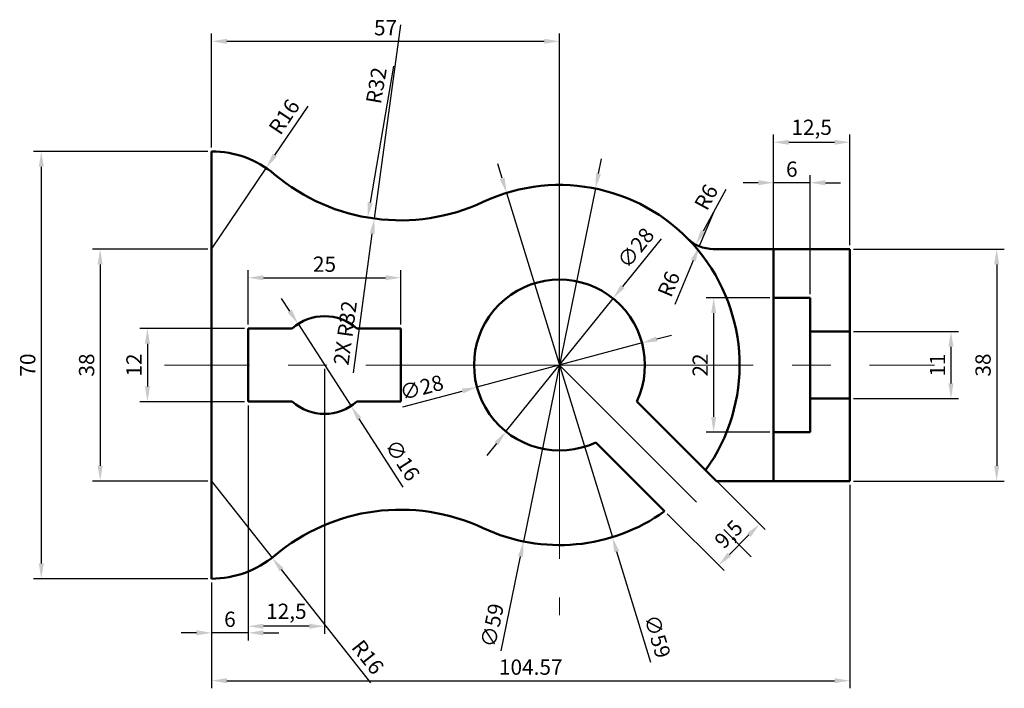
# Model space of a CAD drawing. Units: millimetres. Extents: x 3399 to 3560, y 1676 to 1786.
import ezdxf

# ---------------------------------------------------------------- set-up
doc = ezdxf.new("R2010")
doc.units = ezdxf.units.MM
doc.linetypes.add('CENTER', pattern=[50.8, 31.75, -6.35, 6.35, -6.35])
for name, color, linetype, lineweight in [('M-CNTR', 2, 'CENTER', 18), ('M-DIMS', 6, 'Continuous', 25), ('M-OUTL', 7, 'Continuous', 50)]:
    doc.layers.add(name, color=color, linetype=linetype, lineweight=lineweight)
doc.styles.get("Standard").update_dxf_attribs({"font": 'arial.ttf'})
doc.dimstyles.new('ISO-25', dxfattribs={"dimtxt": 2.5, "dimasz": 2.5, "dimexe": 1.25, "dimexo": 0.625, "dimtad": 1, "dimtxsty": 'Standard', "dimcen": 2.5, "dimadec": 0, "dimazin": 0, "dimtfac": 1, "dimtmove": 0, "dimatfit": 3, "dimfxl": 1, "dimarcsym": 0})

# ---------------------------------------------------------------- blocks, each defined once
blk = doc.blocks.new('*D1')
at = {"layer": 'Defpoints', "color": 0, "transparency": 16777216}
for p in [(3430.34, 1764.16), (3402.43, 1694.16), (3430.34, 1694.16)]:
    blk.add_point(p, dxfattribs=at)
at = {"layer": 'M-DIMS', "color": 0, "lineweight": -2, "transparency": 16777216}
for p, q in [((3429.72, 1764.16), (3401.18, 1764.16)), ((3402.43, 1761.66), (3402.43, 1696.66)), ((3429.72, 1694.16), (3401.18, 1694.16))]:
    blk.add_line(p, q, dxfattribs=at)
at = {"layer": 'M-DIMS', "color": 0, "transparency": 16777216}
for points in [[(3402.02, 1761.66), (3402.85, 1761.66), (3402.43, 1764.16)], [(3402.02, 1696.66), (3402.85, 1696.66), (3402.43, 1694.16)]]:
    blk.add_solid(points, dxfattribs=at)
at = {"layer": 'M-DIMS', "color": 0, "transparency": 16777216, "insert": (3400.53, 1729.16), "char_height": 2.5, "attachment_point": 5, "rotation": 90}
blk.add_mtext('70', dxfattribs=at)
blk = doc.blocks.new('*D2')
at = {"layer": 'Defpoints', "color": 0, "transparency": 16777216}
for p in [(3534.91, 1748.16), (3534.91, 1710.16), (3558.98, 1710.16)]:
    blk.add_point(p, dxfattribs=at)
at = {"layer": 'M-DIMS', "color": 0, "lineweight": -2, "transparency": 16777216}
for p, q in [((3535.53, 1748.16), (3560.23, 1748.16)), ((3558.98, 1745.66), (3558.98, 1712.66)), ((3535.53, 1710.16), (3560.23, 1710.16))]:
    blk.add_line(p, q, dxfattribs=at)
at = {"layer": 'M-DIMS', "color": 0, "transparency": 16777216}
for points in [[(3558.56, 1745.66), (3559.39, 1745.66), (3558.98, 1748.16)], [(3558.56, 1712.66), (3559.39, 1712.66), (3558.98, 1710.16)]]:
    blk.add_solid(points, dxfattribs=at)
at = {"layer": 'M-DIMS', "color": 0, "transparency": 16777216, "insert": (3557.07, 1729.16), "char_height": 2.5, "attachment_point": 5, "rotation": 90}
blk.add_mtext('38', dxfattribs=at)
blk = doc.blocks.new('*D3')
at = {"layer": 'Defpoints', "color": 0, "transparency": 16777216}
for p in [(3534.91, 1734.66), (3534.91, 1723.66), (3551.48, 1723.66)]:
    blk.add_point(p, dxfattribs=at)
at = {"layer": 'M-DIMS', "color": 0, "lineweight": -2, "transparency": 16777216}
for p, q in [((3535.53, 1734.66), (3552.73, 1734.66)), ((3551.48, 1732.16), (3551.48, 1726.16)), ((3535.53, 1723.66), (3552.73, 1723.66))]:
    blk.add_line(p, q, dxfattribs=at)
at = {"layer": 'M-DIMS', "color": 0, "transparency": 16777216}
for points in [[(3551.06, 1732.16), (3551.9, 1732.16), (3551.48, 1734.66)], [(3551.06, 1726.16), (3551.9, 1726.16), (3551.48, 1723.66)]]:
    blk.add_solid(points, dxfattribs=at)
at = {"layer": 'M-DIMS', "color": 0, "transparency": 16777216, "insert": (3549.6, 1729.16), "char_height": 2.5, "attachment_point": 5, "rotation": 90}
blk.add_mtext('11', dxfattribs=at)
blk = doc.blocks.new('*D4')
at = {"layer": 'Defpoints', "color": 0, "transparency": 16777216}
for p in [(3522.41, 1740.16), (3512.6, 1718.16), (3522.41, 1718.16)]:
    blk.add_point(p, dxfattribs=at)
at = {"layer": 'M-DIMS', "color": 0, "lineweight": -2, "transparency": 16777216}
for p, q in [((3521.78, 1740.16), (3511.35, 1740.16)), ((3512.6, 1737.66), (3512.6, 1720.66)), ((3521.78, 1718.16), (3511.35, 1718.16))]:
    blk.add_line(p, q, dxfattribs=at)
at = {"layer": 'M-DIMS', "color": 0, "transparency": 16777216}
for points in [[(3512.19, 1737.66), (3513.02, 1737.66), (3512.6, 1740.16)], [(3512.19, 1720.66), (3513.02, 1720.66), (3512.6, 1718.16)]]:
    blk.add_solid(points, dxfattribs=at)
at = {"layer": 'M-DIMS', "color": 0, "transparency": 16777216, "insert": (3510.72, 1729.16), "char_height": 2.5, "attachment_point": 5, "rotation": 90}
blk.add_mtext('22', dxfattribs=at)
blk = doc.blocks.new('*D5')
at = {"layer": 'Defpoints', "color": 0, "transparency": 16777216}
for p in [(3522.41, 1759.03), (3522.41, 1740.16), (3528.41, 1740.16)]:
    blk.add_point(p, dxfattribs=at)
at = {"layer": 'M-DIMS', "color": 0, "lineweight": -2, "transparency": 16777216}
for p, q in [((3522.41, 1740.79), (3522.41, 1760.28)), ((3528.41, 1740.79), (3528.41, 1760.28)), ((3519.91, 1759.03), (3517.41, 1759.03)), ((3528.41, 1759.03), (3522.41, 1759.03)), ((3530.91, 1759.03), (3533.41, 1759.03))]:
    blk.add_line(p, q, dxfattribs=at)
at = {"layer": 'M-DIMS', "color": 0, "transparency": 16777216}
for points in [[(3519.91, 1759.45), (3519.91, 1758.61), (3522.41, 1759.03)], [(3530.91, 1759.45), (3530.91, 1758.61), (3528.41, 1759.03)]]:
    blk.add_solid(points, dxfattribs=at)
at = {"layer": 'M-DIMS', "color": 0, "transparency": 16777216, "insert": (3525.41, 1760.93), "char_height": 2.5, "attachment_point": 5}
blk.add_mtext('6', dxfattribs=at)
blk = doc.blocks.new('*D6')
at = {"layer": 'Defpoints', "color": 0, "transparency": 16777216}
for p in [(3511.29, 1711.93), (3504.57, 1705.22), (3513.42, 1696.37)]:
    blk.add_point(p, dxfattribs=at)
at = {"layer": 'M-DIMS', "color": 0, "lineweight": -2, "transparency": 16777216}
for p, q in [((3511.73, 1711.49), (3521.02, 1702.2)), ((3505.01, 1704.78), (3514.3, 1695.48)), ((3518.37, 1701.32), (3515.19, 1698.14))]:
    blk.add_line(p, q, dxfattribs=at)
at = {"layer": 'M-DIMS', "color": 0, "transparency": 16777216}
for points in [[(3518.08, 1701.61), (3518.66, 1701.02), (3520.14, 1703.09)], [(3514.89, 1698.43), (3515.48, 1697.84), (3513.42, 1696.37)]]:
    blk.add_solid(points, dxfattribs=at)
at = {"layer": 'M-DIMS', "color": 0, "transparency": 16777216, "insert": (3515.28, 1701.23), "char_height": 2.5, "attachment_point": 5, "rotation": 45}
blk.add_mtext('9,5', dxfattribs=at)
blk = doc.blocks.new('*D7')
at = {"layer": 'Defpoints', "color": 0, "transparency": 16777216}
for p in [(3439.27, 1761.44), (3430.34, 1748.16)]:
    blk.add_point(p, dxfattribs=at)
at = {"layer": 'M-DIMS', "color": 0, "lineweight": -2, "transparency": 16777216}
for p, q in [((3446.09, 1771.58), (3440.66, 1763.52)), ((3430.34, 1748.16), (3439.27, 1761.44))]:
    blk.add_line(p, q, dxfattribs=at)
at = {"layer": 'M-DIMS', "color": 0, "transparency": 16777216}
blk.add_solid([(3440.32, 1763.75), (3441.01, 1763.28), (3439.27, 1761.44)], dxfattribs=at)
at = {"layer": 'M-DIMS', "color": 0, "transparency": 16777216, "insert": (3442.5, 1769.65), "char_height": 2.5, "attachment_point": 5, "rotation": 56.0827}
blk.add_mtext('R16', dxfattribs=at)
blk = doc.blocks.new('*D8')
at = {"layer": 'Defpoints', "color": 0, "transparency": 16777216}
for p in [(3430.34, 1710.16), (3440.25, 1697.6)]:
    blk.add_point(p, dxfattribs=at)
at = {"layer": 'M-DIMS', "color": 0, "lineweight": -2, "transparency": 16777216}
for p, q in [((3430.34, 1710.16), (3440.25, 1697.6)), ((3456.43, 1677.1), (3441.8, 1695.64))]:
    blk.add_line(p, q, dxfattribs=at)
at = {"layer": 'M-DIMS', "color": 0, "transparency": 16777216}
blk.add_solid([(3442.13, 1695.9), (3441.47, 1695.38), (3440.25, 1697.6)], dxfattribs=at)
at = {"layer": 'M-DIMS', "color": 0, "transparency": 16777216, "insert": (3455.69, 1681.11), "char_height": 2.5, "attachment_point": 5, "rotation": 308.2765}
blk.add_mtext('R16', dxfattribs=at)
blk = doc.blocks.new('*D9')
at = {"layer": 'Defpoints', "color": 0, "transparency": 16777216}
for p in [(3461.28, 1784.87), (3455.9, 1753.32)]:
    blk.add_point(p, dxfattribs=at)
at = {"layer": 'M-DIMS', "color": 0, "lineweight": -2, "transparency": 16777216}
blk.add_line((3460.13, 1778.13), (3456.32, 1755.79), dxfattribs=at)
at = {"layer": 'M-DIMS', "color": 0, "transparency": 16777216}
blk.add_solid([(3455.91, 1755.86), (3456.73, 1755.72), (3455.9, 1753.32)], dxfattribs=at)
at = {"layer": 'M-DIMS', "color": 0, "transparency": 16777216, "insert": (3457.65, 1774.9), "char_height": 2.5, "attachment_point": 5, "rotation": 80.3303}
blk.add_mtext('R32', dxfattribs=at)
blk = doc.blocks.new('*D10')
at = {"layer": 'Defpoints', "color": 0, "transparency": 16777216}
for p in [(3512.55, 1754.16), (3509.67, 1748.9)]:
    blk.add_point(p, dxfattribs=at)
at = {"layer": 'M-DIMS', "color": 0, "lineweight": -2, "transparency": 16777216}
blk.add_line((3514.6, 1757.92), (3510.87, 1751.09), dxfattribs=at)
at = {"layer": 'M-DIMS', "color": 0, "transparency": 16777216}
blk.add_solid([(3510.5, 1751.29), (3511.23, 1750.89), (3509.67, 1748.9)], dxfattribs=at)
at = {"layer": 'M-DIMS', "color": 0, "transparency": 16777216, "insert": (3511.66, 1756.51), "char_height": 2.5, "attachment_point": 5, "rotation": 61.3621}
blk.add_mtext('R6', dxfattribs=at)
blk = doc.blocks.new('*D11')
at = {"layer": 'Defpoints', "color": 0, "transparency": 16777216}
for p in [(3444.51, 1735.89), (3453.18, 1722.44)]:
    blk.add_point(p, dxfattribs=at)
at = {"layer": 'M-DIMS', "color": 0, "lineweight": -2, "transparency": 16777216}
for p, q in [((3443.15, 1737.99), (3441.8, 1740.09)), ((3444.51, 1735.89), (3453.18, 1722.44)), ((3461.73, 1709.17), (3454.53, 1720.34))]:
    blk.add_line(p, q, dxfattribs=at)
at = {"layer": 'M-DIMS', "color": 0, "transparency": 16777216}
for points in [[(3443.5, 1738.21), (3442.8, 1737.76), (3444.51, 1735.89)], [(3454.88, 1720.56), (3454.18, 1720.11), (3453.18, 1722.44)]]:
    blk.add_solid(points, dxfattribs=at)
at = {"layer": 'M-DIMS', "color": 0, "transparency": 16777216, "insert": (3461.34, 1713.41), "char_height": 2.5, "attachment_point": 5, "rotation": 302.8035}
blk.add_mtext('∅16', dxfattribs=at)
blk = doc.blocks.new('*D12')
at = {"layer": 'Defpoints', "color": 0, "transparency": 16777216}
for p in [(3496.11, 1740.07), (3478.57, 1718.25)]:
    blk.add_point(p, dxfattribs=at)
at = {"layer": 'M-DIMS', "color": 0, "lineweight": -2, "transparency": 16777216}
for p, q in [((3503.98, 1749.86), (3497.68, 1742.02)), ((3478.57, 1718.25), (3496.11, 1740.07)), ((3477, 1716.3), (3475.44, 1714.36))]:
    blk.add_line(p, q, dxfattribs=at)
at = {"layer": 'M-DIMS', "color": 0, "transparency": 16777216}
for points in [[(3497.36, 1742.28), (3498.01, 1741.76), (3496.11, 1740.07)], [(3476.68, 1716.57), (3477.33, 1716.04), (3478.57, 1718.25)]]:
    blk.add_solid(points, dxfattribs=at)
at = {"layer": 'M-DIMS', "color": 0, "transparency": 16777216, "insert": (3500.08, 1748.15), "char_height": 2.5, "attachment_point": 5, "rotation": 51.2016}
blk.add_mtext('∅28', dxfattribs=at)
blk = doc.blocks.new('*D13')
at = {"layer": 'Defpoints', "color": 0, "transparency": 16777216}
for p in [(3493.23, 1758.07), (3481.46, 1700.26)]:
    blk.add_point(p, dxfattribs=at)
at = {"layer": 'M-DIMS', "color": 0, "lineweight": -2, "transparency": 16777216}
for p, q in [((3493.73, 1760.52), (3494.22, 1762.97)), ((3493.23, 1758.07), (3481.46, 1700.26)), ((3477.81, 1682.36), (3480.96, 1697.81))]:
    blk.add_line(p, q, dxfattribs=at)
at = {"layer": 'M-DIMS', "color": 0, "transparency": 16777216}
for points in [[(3493.32, 1760.6), (3494.13, 1760.44), (3493.23, 1758.07)], [(3480.55, 1697.89), (3481.37, 1697.72), (3481.46, 1700.26)]]:
    blk.add_solid(points, dxfattribs=at)
at = {"layer": 'M-DIMS', "color": 0, "transparency": 16777216, "insert": (3476.63, 1686.45), "char_height": 2.5, "attachment_point": 5, "rotation": 78.4924}
blk.add_mtext('∅59', dxfattribs=at)
blk = doc.blocks.new('*D14')
at = {"layer": 'Defpoints', "color": 0, "transparency": 16777216}
for p in [(3461.34, 1743.46), (3436.34, 1735.16), (3461.34, 1735.16)]:
    blk.add_point(p, dxfattribs=at)
at = {"layer": 'M-DIMS', "color": 0, "lineweight": -2, "transparency": 16777216}
for p, q in [((3436.34, 1735.79), (3436.34, 1744.71)), ((3461.34, 1735.79), (3461.34, 1744.71)), ((3438.84, 1743.46), (3458.84, 1743.46))]:
    blk.add_line(p, q, dxfattribs=at)
at = {"layer": 'M-DIMS', "color": 0, "transparency": 16777216}
for points in [[(3438.84, 1743.88), (3438.84, 1743.04), (3436.34, 1743.46)], [(3458.84, 1743.88), (3458.84, 1743.04), (3461.34, 1743.46)]]:
    blk.add_solid(points, dxfattribs=at)
at = {"layer": 'M-DIMS', "color": 0, "transparency": 16777216, "insert": (3448.84, 1745.36), "char_height": 2.5, "attachment_point": 5}
blk.add_mtext('25', dxfattribs=at)
blk = doc.blocks.new('*D15')
at = {"layer": 'Defpoints', "color": 0, "transparency": 16777216}
for p in [(3430.34, 1748.16), (3412.08, 1710.16), (3430.34, 1710.16)]:
    blk.add_point(p, dxfattribs=at)
at = {"layer": 'M-DIMS', "color": 0, "lineweight": -2, "transparency": 16777216}
for p, q in [((3429.72, 1748.16), (3410.83, 1748.16)), ((3412.08, 1745.66), (3412.08, 1712.66)), ((3429.72, 1710.16), (3410.83, 1710.16))]:
    blk.add_line(p, q, dxfattribs=at)
at = {"layer": 'M-DIMS', "color": 0, "transparency": 16777216}
for points in [[(3411.66, 1745.66), (3412.49, 1745.66), (3412.08, 1748.16)], [(3411.66, 1712.66), (3412.49, 1712.66), (3412.08, 1710.16)]]:
    blk.add_solid(points, dxfattribs=at)
at = {"layer": 'M-DIMS', "color": 0, "transparency": 16777216, "insert": (3410.18, 1729.16), "char_height": 2.5, "attachment_point": 5, "rotation": 90}
blk.add_mtext('38', dxfattribs=at)
blk = doc.blocks.new('*D16')
at = {"layer": 'Defpoints', "color": 0, "transparency": 16777216}
for p in [(3436.34, 1735.16), (3419.82, 1723.16), (3436.34, 1723.16)]:
    blk.add_point(p, dxfattribs=at)
at = {"layer": 'M-DIMS', "color": 0, "lineweight": -2, "transparency": 16777216}
for p, q in [((3435.72, 1735.16), (3418.57, 1735.16)), ((3419.82, 1732.66), (3419.82, 1725.66)), ((3435.72, 1723.16), (3418.57, 1723.16))]:
    blk.add_line(p, q, dxfattribs=at)
at = {"layer": 'M-DIMS', "color": 0, "transparency": 16777216}
for points in [[(3419.41, 1732.66), (3420.24, 1732.66), (3419.82, 1735.16)], [(3419.41, 1725.66), (3420.24, 1725.66), (3419.82, 1723.16)]]:
    blk.add_solid(points, dxfattribs=at)
at = {"layer": 'M-DIMS', "color": 0, "transparency": 16777216, "insert": (3417.94, 1729.16), "char_height": 2.5, "attachment_point": 5, "rotation": 90}
blk.add_mtext('12', dxfattribs=at)
blk = doc.blocks.new('*D17')
at = {"layer": 'Defpoints', "color": 0, "transparency": 16777216}
for p in [(3487.34, 1782.2), (3430.34, 1764.16), (3487.34, 1729.16)]:
    blk.add_point(p, dxfattribs=at)
at = {"layer": 'M-DIMS', "color": 0, "lineweight": -2, "transparency": 16777216}
for p, q in [((3430.34, 1764.79), (3430.34, 1783.45)), ((3487.34, 1729.79), (3487.34, 1783.45)), ((3432.84, 1782.2), (3484.84, 1782.2))]:
    blk.add_line(p, q, dxfattribs=at)
at = {"layer": 'M-DIMS', "color": 0, "transparency": 16777216}
for points in [[(3432.84, 1782.62), (3432.84, 1781.78), (3430.34, 1782.2)], [(3484.84, 1782.62), (3484.84, 1781.78), (3487.34, 1782.2)]]:
    blk.add_solid(points, dxfattribs=at)
at = {"layer": 'M-DIMS', "color": 0, "transparency": 16777216, "insert": (3458.84, 1784.1), "char_height": 2.5, "attachment_point": 5}
blk.add_mtext('57', dxfattribs=at)
blk = doc.blocks.new('*D18')
at = {"layer": 'Defpoints', "color": 0, "transparency": 16777216}
for p in [(3436.34, 1723.16), (3430.34, 1694.16), (3430.34, 1685.29)]:
    blk.add_point(p, dxfattribs=at)
at = {"layer": 'M-DIMS', "color": 0, "lineweight": -2, "transparency": 16777216}
for p, q in [((3436.34, 1722.54), (3436.34, 1684.04)), ((3430.34, 1693.54), (3430.34, 1684.04)), ((3427.84, 1685.29), (3425.34, 1685.29)), ((3436.34, 1685.29), (3430.34, 1685.29)), ((3438.84, 1685.29), (3441.34, 1685.29))]:
    blk.add_line(p, q, dxfattribs=at)
at = {"layer": 'M-DIMS', "color": 0, "transparency": 16777216}
for points in [[(3427.84, 1685.71), (3427.84, 1684.88), (3430.34, 1685.29)], [(3438.84, 1685.71), (3438.84, 1684.88), (3436.34, 1685.29)]]:
    blk.add_solid(points, dxfattribs=at)
at = {"layer": 'M-DIMS', "color": 0, "transparency": 16777216, "insert": (3433.34, 1687.19), "char_height": 2.5, "attachment_point": 5}
blk.add_mtext('6', dxfattribs=at)
blk = doc.blocks.new('*D19')
at = {"layer": 'Defpoints', "color": 0, "transparency": 16777216}
for p in [(3448.84, 1729.16), (3436.34, 1723.16), (3436.34, 1686.37)]:
    blk.add_point(p, dxfattribs=at)
at = {"layer": 'M-DIMS', "color": 0, "lineweight": -2, "transparency": 16777216}
for p, q in [((3448.84, 1728.54), (3448.84, 1685.12)), ((3436.34, 1722.54), (3436.34, 1685.12)), ((3446.34, 1686.37), (3438.84, 1686.37))]:
    blk.add_line(p, q, dxfattribs=at)
at = {"layer": 'M-DIMS', "color": 0, "transparency": 16777216}
for points in [[(3438.84, 1686.79), (3438.84, 1685.95), (3436.34, 1686.37)], [(3446.34, 1686.79), (3446.34, 1685.95), (3448.84, 1686.37)]]:
    blk.add_solid(points, dxfattribs=at)
at = {"layer": 'M-DIMS', "color": 0, "transparency": 16777216, "insert": (3442.59, 1688.5), "char_height": 2.5, "attachment_point": 5}
blk.add_mtext('12,5', dxfattribs=at)
blk = doc.blocks.new('*D20')
at = {"layer": 'Defpoints', "color": 0, "transparency": 16777216}
for p in [(3534.91, 1765.66), (3534.91, 1748.16), (3522.41, 1740.16)]:
    blk.add_point(p, dxfattribs=at)
at = {"layer": 'M-DIMS', "color": 0, "lineweight": -2, "transparency": 16777216}
for p, q in [((3522.41, 1740.79), (3522.41, 1766.91)), ((3534.91, 1748.79), (3534.91, 1766.91)), ((3524.91, 1765.66), (3532.41, 1765.66))]:
    blk.add_line(p, q, dxfattribs=at)
at = {"layer": 'M-DIMS', "color": 0, "transparency": 16777216}
for points in [[(3524.91, 1766.07), (3524.91, 1765.24), (3522.41, 1765.66)], [(3532.41, 1766.07), (3532.41, 1765.24), (3534.91, 1765.66)]]:
    blk.add_solid(points, dxfattribs=at)
at = {"layer": 'M-DIMS', "color": 0, "transparency": 16777216, "insert": (3528.66, 1767.79), "char_height": 2.5, "attachment_point": 5}
blk.add_mtext('12,5', dxfattribs=at)
blk = doc.blocks.new('*D21')
at = {"layer": 'Defpoints', "color": 0, "transparency": 16777216}
for p in [(3534.91, 1710.16), (3430.34, 1694.16), (3534.91, 1677.45)]:
    blk.add_point(p, dxfattribs=at)
at = {"layer": 'M-DIMS', "color": 0, "lineweight": -2, "transparency": 16777216}
for p, q in [((3534.91, 1709.54), (3534.91, 1676.2)), ((3430.34, 1693.54), (3430.34, 1676.2)), ((3432.84, 1677.45), (3532.41, 1677.45))]:
    blk.add_line(p, q, dxfattribs=at)
at = {"layer": 'M-DIMS', "color": 0, "transparency": 16777216}
for points in [[(3432.84, 1677.87), (3432.84, 1677.04), (3430.34, 1677.45)], [(3532.41, 1677.87), (3532.41, 1677.04), (3534.91, 1677.45)]]:
    blk.add_solid(points, dxfattribs=at)
at = {"layer": 'M-DIMS', "color": 0, "transparency": 16777216, "insert": (3482.63, 1679.35), "char_height": 2.5, "attachment_point": 5}
blk.add_mtext('104.57', dxfattribs=at)
blk = doc.blocks.new('*D22')
at = {"layer": 'Defpoints', "color": 0, "transparency": 16777216}
for p in [(3478.68, 1757.36), (3496, 1700.96)]:
    blk.add_point(p, dxfattribs=at)
at = {"layer": 'M-DIMS', "color": 0, "lineweight": -2, "transparency": 16777216}
for p, q in [((3477.95, 1759.75), (3477.22, 1762.14)), ((3478.68, 1757.36), (3496, 1700.96)), ((3502.3, 1680.43), (3496.73, 1698.57))]:
    blk.add_line(p, q, dxfattribs=at)
at = {"layer": 'M-DIMS', "color": 0, "transparency": 16777216}
for points in [[(3478.35, 1759.88), (3477.55, 1759.63), (3478.68, 1757.36)], [(3497.13, 1698.69), (3496.33, 1698.45), (3496, 1700.96)]]:
    blk.add_solid(points, dxfattribs=at)
at = {"layer": 'M-DIMS', "color": 0, "transparency": 16777216, "insert": (3503.08, 1684.62), "char_height": 2.5, "attachment_point": 5, "rotation": 287.0655}
blk.add_mtext('∅59', dxfattribs=at)
blk = doc.blocks.new('*D23')
at = {"layer": 'Defpoints', "color": 0, "transparency": 16777216}
for p in [(3500.87, 1732.79), (3473.82, 1725.54)]:
    blk.add_point(p, dxfattribs=at)
at = {"layer": 'M-DIMS', "color": 0, "lineweight": -2, "transparency": 16777216}
for p, q in [((3500.87, 1732.79), (3473.82, 1725.54)), ((3503.28, 1733.43), (3505.69, 1734.08)), ((3461.69, 1722.29), (3471.4, 1724.89))]:
    blk.add_line(p, q, dxfattribs=at)
at = {"layer": 'M-DIMS', "color": 0, "transparency": 16777216}
for points in [[(3503.17, 1733.84), (3503.39, 1733.03), (3500.87, 1732.79)], [(3471.3, 1725.3), (3471.51, 1724.49), (3473.82, 1725.54)]]:
    blk.add_solid(points, dxfattribs=at)
at = {"layer": 'M-DIMS', "color": 0, "transparency": 16777216, "insert": (3464.83, 1725.17), "char_height": 2.5, "attachment_point": 5, "rotation": 14.9994}
blk.add_mtext('∅28', dxfattribs=at)
blk = doc.blocks.new('*D24')
at = {"layer": 'Defpoints', "color": 0, "transparency": 16777216}
for p in [(3461.28, 1784.87), (3457, 1753.15)]:
    blk.add_point(p, dxfattribs=at)
at = {"layer": 'M-DIMS', "color": 0, "lineweight": -2, "transparency": 16777216}
for p, q in [((3461.28, 1784.87), (3457, 1753.15)), ((3453.59, 1727.88), (3456.66, 1750.68))]:
    blk.add_line(p, q, dxfattribs=at)
at = {"layer": 'M-DIMS', "color": 0, "transparency": 16777216}
blk.add_solid([(3456.25, 1750.73), (3457.08, 1750.62), (3457, 1753.15)], dxfattribs=at)
at = {"layer": 'M-DIMS', "color": 0, "transparency": 16777216, "insert": (3452.55, 1734.38), "char_height": 2.5, "attachment_point": 5, "rotation": 82.3171}
blk.add_mtext('2X R32', dxfattribs=at)
blk = doc.blocks.new('*D25')
at = {"layer": 'Defpoints', "color": 0, "transparency": 16777216}
for p in [(3512.55, 1754.16), (3510.24, 1748.62)]:
    blk.add_point(p, dxfattribs=at)
at = {"layer": 'M-DIMS', "color": 0, "lineweight": -2, "transparency": 16777216}
for p, q in [((3512.55, 1754.16), (3510.24, 1748.62)), ((3506.29, 1739.14), (3509.28, 1746.32))]:
    blk.add_line(p, q, dxfattribs=at)
at = {"layer": 'M-DIMS', "color": 0, "transparency": 16777216}
blk.add_solid([(3508.89, 1746.48), (3509.66, 1746.16), (3510.24, 1748.62)], dxfattribs=at)
at = {"layer": 'M-DIMS', "color": 0, "transparency": 16777216, "insert": (3505.55, 1742.3), "char_height": 2.5, "attachment_point": 5, "rotation": 67.3845}
blk.add_mtext('R6', dxfattribs=at)

msp = doc.modelspace()

# ---------------------------------------------------------------- linework, layer by layer
at = {"layer": 'M-CNTR'}
for p, q in [((3487.342, 1729.164), (3487.342, 1768.619)), ((3430.342, 1729.164), (3422.595, 1729.164)), ((3487.342, 1729.164), (3430.342, 1729.164)), ((3487.342, 1729.164), (3521.362, 1695.143)), ((3487.342, 1729.164), (3548.781, 1729.164)), ((3487.342, 1729.164), (3487.342, 1688.203))]:
    msp.add_line(p, q, dxfattribs=at)
at = {"layer": 'M-OUTL'}
for p, q in [((3430.342, 1729.164), (3430.342, 1764.164)), ((3512.546, 1748.164), (3534.909, 1748.164)), ((3522.409, 1748.164), (3522.409, 1710.164)), ((3534.909, 1748.164), (3534.909, 1710.164)), ((3522.409, 1740.164), (3528.409, 1740.164)), ((3528.409, 1740.164), (3528.409, 1718.164)), ((3436.342, 1729.164), (3436.342, 1735.164)), ((3436.342, 1735.164), (3443.551, 1735.164)), ((3454.134, 1735.164), (3461.342, 1735.164)), ((3461.342, 1735.164), (3461.342, 1723.164)), ((3528.409, 1734.664), (3534.909, 1734.664)), ((3534.909, 1734.664), (3534.909, 1723.664)), ((3430.342, 1729.164), (3430.342, 1694.164)), ((3436.342, 1723.164), (3436.342, 1729.164)), ((3443.551, 1723.164), (3436.342, 1723.164)), ((3461.342, 1723.164), (3454.134, 1723.164)), ((3500.013, 1723.21), (3513.06, 1710.164)), ((3534.909, 1723.664), (3528.409, 1723.664)), ((3528.409, 1718.164), (3522.409, 1718.164)), ((3493.296, 1716.492), (3504.571, 1705.217)), ((3430.342, 1694.164), (3430.342, 1710.164)), ((3534.909, 1710.164), (3513.06, 1710.164))]:
    msp.add_line(p, q, dxfattribs=at)
for centre, radius, start, end in [((3430.342, 1748.164), 16, 49.87518, 90), ((3461.276, 1784.866), 32, 229.87518, 295.07726), ((3487.342, 1729.164), 29.5, 324.26593, 115.07726), ((3512.546, 1754.164), 6, 224.767, 270), ((3487.342, 1729.164), 14, 334.83336, 295.16664), ((3448.842, 1729.164), 8, 48.59038, 131.40962), ((3448.842, 1729.164), 8, 228.59038, 311.40962), ((3461.276, 1673.461), 32, 64.92274, 130.12482), ((3487.342, 1729.164), 29.5, 244.92274, 305.73407), ((3430.342, 1710.164), 16, 270, 310.12482)]:
    msp.add_arc(centre, radius, start, end, dxfattribs=at)

# ---------------------------------------------------------------- dimensions: what is measured, and where the dimension line sits
at = {"layer": 'M-DIMS'}
for base, p1, p2, override, picture, middle in [((3487.342, 1782.201), (3430.342, 1764.164), (3487.342, 1729.164), {"dimclrd": 0, "dimclre": 0, "dimclrt": 0}, '*D17', (3458.842, 1784.097)), ((3534.909, 1765.658), (3522.409, 1740.164), (3534.909, 1748.164), {"dimclrd": 0, "dimclre": 0, "dimclrt": 0}, '*D20', (3528.659, 1767.786)), ((3522.409, 1759.029), (3528.409, 1740.164), (3522.409, 1740.164), {"dimclrd": 0, "dimclre": 0, "dimclrt": 0}, '*D5', (3525.409, 1760.931)), ((3461.342, 1743.461), (3436.342, 1735.164), (3461.342, 1735.164), {"dimclrd": 0, "dimclre": 0, "dimclrt": 0}, '*D14', (3448.842, 1745.362)), ((3436.342, 1686.369), (3448.842, 1729.164), (3436.342, 1723.164), {"dimclrd": 0, "dimclre": 0, "dimclrt": 0}, '*D19', (3442.592, 1688.496)), ((3430.342, 1685.293), (3436.342, 1723.164), (3430.342, 1694.164), {"dimclrd": 0, "dimclre": 0, "dimclrt": 0}, '*D18', (3433.342, 1687.195)), ((3534.909, 1677.453), (3430.342, 1694.164), (3534.909, 1710.164), {"dimdec": 2, "dimlfac": 1, "dimrnd": 0, "dimzin": 0, "dimdsep": 46, "dimlunit": 2}, '*D21', (3482.625, 1679.354))]:
    dim = msp.add_linear_dim(base=base, p1=p1, p2=p2, dimstyle='ISO-25', override=override, dxfattribs=at)
    dim.commit()
    dim.dimension.update_dxf_attribs({"geometry": picture, "text_midpoint": middle})
dim = msp.add_radius_dim(center=(3461.276, 1784.866), mpoint=(3456.998, 1753.154), text='2X <>', dimstyle='ISO-25', override={"dimdec": 0, "dimlfac": 1, "dimrnd": 0, "dimzin": 0, "dimdsep": 46, "dimlunit": 2}, dxfattribs=at)
dim.commit()
dim.dimension.update_dxf_attribs({"geometry": '*D24', "text_midpoint": (3454.431, 1734.126), "dimtype": 164})
for center, mpoint, picture, middle in [((3461.276, 1784.866), (3455.901, 1753.321), '*D9', (3459.523, 1774.581)), ((3512.546, 1754.164), (3509.671, 1748.898), '*D10', (3513.332, 1755.603)), ((3430.342, 1710.164), (3440.253, 1697.603), '*D8', (3454.198, 1679.931))]:
    dim = msp.add_radius_dim(center=center, mpoint=mpoint, dimstyle='ISO-25', override={"dimclrd": 0, "dimclre": 0, "dimclrt": 0}, dxfattribs=at)
    dim.commit()
    dim.dimension.update_dxf_attribs({"geometry": picture, "text_midpoint": middle, "dimtype": 164})
for center, mpoint, override, picture, middle in [((3430.342, 1748.164), (3439.27, 1761.441), {"dimclrd": 0, "dimclre": 0, "dimclrt": 0}, '*D7', (3442.497, 1769.648)), ((3512.546, 1754.164), (3510.239, 1748.625), {"dimdec": 0, "dimlfac": 1, "dimrnd": 0, "dimzin": 0, "dimdsep": 46, "dimlunit": 2}, '*D25', (3505.546, 1742.304))]:
    dim = msp.add_radius_dim(center=center, mpoint=mpoint, dimstyle='ISO-25', override=override, dxfattribs=at)
    dim.commit()
    dim.dimension.update_dxf_attribs({"geometry": picture, "text_midpoint": middle})
for base, p1, p2, picture, middle in [((3402.434, 1694.164), (3430.342, 1764.164), (3430.342, 1694.164), '*D1', (3400.533, 1729.164)), ((3412.077, 1710.164), (3430.342, 1748.164), (3430.342, 1710.164), '*D15', (3410.175, 1729.164)), ((3558.977, 1710.164), (3534.909, 1748.164), (3534.909, 1710.164), '*D2', (3557.074, 1729.164)), ((3512.602, 1718.164), (3522.409, 1740.164), (3522.409, 1718.164), '*D4', (3510.722, 1729.164)), ((3419.824, 1723.164), (3436.342, 1735.164), (3436.342, 1723.164), '*D16', (3417.943, 1729.164)), ((3551.481, 1723.664), (3534.909, 1734.664), (3534.909, 1723.664), '*D3', (3549.601, 1729.164))]:
    dim = msp.add_linear_dim(base=base, p1=p1, p2=p2, angle=90, dimstyle='ISO-25', override={"dimclrd": 0, "dimclre": 0, "dimclrt": 0}, dxfattribs=at)
    dim.commit()
    dim.dimension.update_dxf_attribs({"geometry": picture, "text_midpoint": middle})
for p1, p2, override, picture, middle in [((3493.227, 1758.071), (3481.457, 1700.257), {"dimclrd": 0, "dimclre": 0, "dimclrt": 0}, '*D13', (3478.566, 1686.059)), ((3478.685, 1757.365), (3495.999, 1700.962), {"dimdec": 0, "dimlfac": 1, "dimrnd": 0, "dimzin": 0, "dimdsep": 46, "dimlunit": 2}, '*D22', (3501.194, 1684.042)), ((3444.508, 1735.888), (3453.176, 1722.439), {"dimclrd": 0, "dimclre": 0, "dimclrt": 0}, '*D11', (3459.685, 1712.341)), ((3500.865, 1732.787), (3473.819, 1725.54), {"dimdec": 0, "dimlfac": 1, "dimrnd": 0, "dimzin": 0, "dimdsep": 46, "dimlunit": 2}, '*D23', (3465.34, 1723.268))]:
    dim = msp.add_diameter_dim_2p(p1=p1, p2=p2, dimstyle='ISO-25', override=override, dxfattribs=at)
    dim.commit()
    dim.dimension.update_dxf_attribs({"geometry": picture, "text_midpoint": middle, "dimtype": 163})
dim = msp.add_diameter_dim_2p(p1=(3478.57, 1718.253), p2=(3496.114, 1740.075), dimstyle='ISO-25', override={"dimclrd": 0, "dimclre": 0, "dimclrt": 0}, dxfattribs=at)
dim.commit()
dim.dimension.update_dxf_attribs({"geometry": '*D12', "text_midpoint": (3500.078, 1748.151)})
dim = msp.add_aligned_dim(p1=(3511.288, 1711.935), p2=(3504.571, 1705.217), distance=12.515, dimstyle='ISO-25', override={"dimclrd": 0, "dimclre": 0, "dimclrt": 0}, dxfattribs=at)
dim.commit()
dim.dimension.update_dxf_attribs({"geometry": '*D6', "text_midpoint": (3515.275, 1701.231)})

doc.saveas('drawing.dxf')
